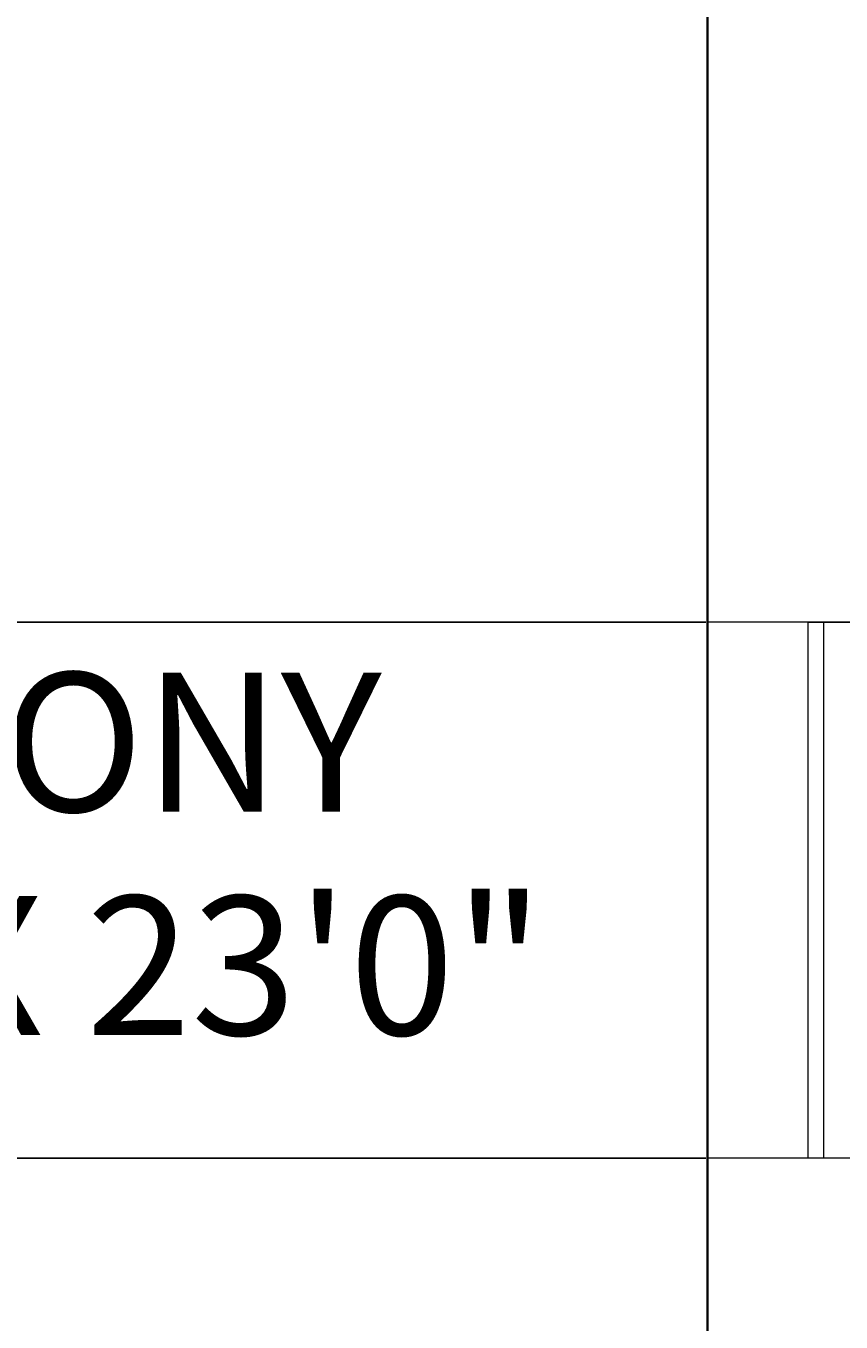
# Model space of a CAD drawing. Units: inches. Extents: x -61 to 1599, y -1316 to 257.
# Tile 58 of 204: x 48 to 85, y -282 to -224. Entities that reach past the tile are written whole.
import ezdxf

# ---------------------------------------------------------------- set-up
doc = ezdxf.new("R2010")
doc.units = ezdxf.units.IN
doc.header["$MEASUREMENT"] = 0
for name, color, linetype, lineweight in [('A-ANNO-DIMS', 2, 'Continuous', 18), ('A-AREA-IDEN', 1, 'Continuous', 18), ('WALLS', 4, 'Continuous', 35), ('WINDOWS', 220, 'Continuous', 18)]:
    doc.layers.add(name, color=color, linetype=linetype, lineweight=lineweight)
doc.styles.get("Standard").update_dxf_attribs({"font": 'arial.ttf'})
doc.dimstyles.get("Standard").update_dxf_attribs({"dimtxt": 0.18, "dimasz": 0.18, "dimexe": 0.18, "dimexo": 0.0625, "dimgap": 0.09, "dimtad": 0, "dimtih": 1, "dimtoh": 1, "dimdec": 0, "dimzin": 0, "dimdsep": 46, "dimlunit": 3, "dimtxsty": 'Standard', "dimcen": 0.09, "dimadec": 0, "dimazin": 0, "dimtfac": 1, "dimtdec": 0, "dimtofl": 0, "dimtmove": 0, "dimatfit": 3, "dimfxl": 1, "dimtolj": 1, "dimtzin": 0, "dimarcsym": 0})

# ---------------------------------------------------------------- blocks, each defined once
blk = doc.blocks.new('WIN-24IN')
for p, q in [((0, 4.5), (0, 9)), ((0, 9), (0, 0)), ((24, 9), (24, 0)), ((0, 5.192), (24, 5.192)), ((0, 4.5), (24, 4.5))]:
    blk.add_line(p, q)
blk = doc.blocks.new('*D687')
at = {"layer": 'A-ANNO-DIMS', "color": 0, "lineweight": -2, "transparency": 16777216}
for p, q in [((289.418, 181.677), (-61.077, 181.677)), ((-60.897, 181.497), (-60.897, -528.952)), ((-60.897, -1239.765), (-60.897, -529.316)), ((319.64, -1239.945), (-61.077, -1239.945))]:
    blk.add_line(p, q, dxfattribs=at)
at = {"layer": 'A-ANNO-DIMS', "color": 0, "transparency": 16777216}
for points in [[(-60.927, 181.497), (-60.867, 181.497), (-60.897, 181.677)], [(-60.927, -1239.765), (-60.867, -1239.765), (-60.897, -1239.945)]]:
    blk.add_solid(points, dxfattribs=at)
at = {"layer": 'DEFPOINTS', "color": 0, "transparency": 16777216}
for p in [(289.481, 181.677), (-60.897, -1239.945), (319.703, -1239.945)]:
    blk.add_point(p, dxfattribs=at)
at = {"layer": 'A-ANNO-DIMS', "color": 0, "transparency": 16777216, "insert": (-60.897, -529.134), "char_height": 0.18, "attachment_point": 5}
blk.add_mtext('\\A1;1421.6', dxfattribs=at)
blk = doc.blocks.new('*D699')
at = {"layer": 'A-ANNO-DIMS', "color": 0, "lineweight": -2, "transparency": 16777216}
for p, q in [((835.64, -167.169), (-61.077, -167.169)), ((-60.897, -167.349), (-60.897, -306.726)), ((-60.897, -446.466), (-60.897, -307.09)), ((841.64, -446.646), (-61.077, -446.646))]:
    blk.add_line(p, q, dxfattribs=at)
at = {"layer": 'A-ANNO-DIMS', "color": 0, "transparency": 16777216}
for points in [[(-60.927, -167.349), (-60.867, -167.349), (-60.897, -167.169)], [(-60.927, -446.466), (-60.867, -446.466), (-60.897, -446.646)]]:
    blk.add_solid(points, dxfattribs=at)
at = {"layer": 'DEFPOINTS', "color": 0, "transparency": 16777216}
for p in [(835.703, -167.169), (-60.897, -446.646), (841.703, -446.646)]:
    blk.add_point(p, dxfattribs=at)
at = {"layer": 'A-ANNO-DIMS', "color": 0, "transparency": 16777216, "insert": (-60.897, -306.908), "char_height": 0.18, "attachment_point": 5}
blk.add_mtext('\\A1;279.5', dxfattribs=at)
blk = doc.blocks.new('*D700')
at = {"layer": 'A-ANNO-DIMS', "color": 0, "lineweight": -2, "transparency": 16777216}
for p, q in [((14.703, -616.882), (14.703, 257.457)), ((14.883, 257.277), (96.772, 257.277)), ((179.572, 257.277), (97.683, 257.277)), ((179.752, -616.882), (179.752, 257.457))]:
    blk.add_line(p, q, dxfattribs=at)
at = {"layer": 'A-ANNO-DIMS', "color": 0, "transparency": 16777216}
for points in [[(14.883, 257.307), (14.883, 257.247), (14.703, 257.277)], [(179.572, 257.307), (179.572, 257.247), (179.752, 257.277)]]:
    blk.add_solid(points, dxfattribs=at)
at = {"layer": 'DEFPOINTS', "color": 0, "transparency": 16777216}
for p in [(179.752, 257.277), (14.703, -616.945), (179.752, -616.945)]:
    blk.add_point(p, dxfattribs=at)
at = {"layer": 'A-ANNO-DIMS', "color": 0, "transparency": 16777216, "insert": (97.227, 257.277), "char_height": 0.18, "attachment_point": 5}
blk.add_mtext('\\A1;165.05', dxfattribs=at)
blk = doc.blocks.new('*D706')
at = {"layer": 'A-ANNO-DIMS', "color": 0, "lineweight": -2, "transparency": 16777216}
for p, q in [((78.64, -175.323), (-61.077, -175.323)), ((-60.897, -175.503), (-60.897, -212.976)), ((-60.897, -250.814), (-60.897, -213.34)), ((78.64, -250.994), (-61.077, -250.994))]:
    blk.add_line(p, q, dxfattribs=at)
at = {"layer": 'A-ANNO-DIMS', "color": 0, "transparency": 16777216}
for points in [[(-60.927, -175.503), (-60.867, -175.503), (-60.897, -175.323)], [(-60.927, -250.814), (-60.867, -250.814), (-60.897, -250.994)]]:
    blk.add_solid(points, dxfattribs=at)
at = {"layer": 'DEFPOINTS', "color": 0, "transparency": 16777216}
for p in [(-60.897, -175.323), (78.703, -175.323), (78.703, -250.994)]:
    blk.add_point(p, dxfattribs=at)
at = {"layer": 'A-ANNO-DIMS', "color": 0, "transparency": 16777216, "insert": (-60.897, -213.158), "char_height": 0.18, "attachment_point": 5}
blk.add_mtext('\\A1;75.67', dxfattribs=at)
blk = doc.blocks.new('*D707')
at = {"layer": 'A-ANNO-DIMS', "color": 0, "lineweight": -2, "transparency": 16777216}
for p, q in [((78.64, -274.994), (-61.077, -274.994)), ((-60.897, -275.174), (-60.897, -308.474)), ((-60.897, -342.139), (-60.897, -308.838)), ((78.64, -342.319), (-61.077, -342.319))]:
    blk.add_line(p, q, dxfattribs=at)
at = {"layer": 'A-ANNO-DIMS', "color": 0, "transparency": 16777216}
for points in [[(-60.927, -275.174), (-60.867, -275.174), (-60.897, -274.994)], [(-60.927, -342.139), (-60.867, -342.139), (-60.897, -342.319)]]:
    blk.add_solid(points, dxfattribs=at)
at = {"layer": 'DEFPOINTS', "color": 0, "transparency": 16777216}
for p in [(78.703, -274.994), (-60.897, -342.319), (78.703, -342.319)]:
    blk.add_point(p, dxfattribs=at)
at = {"layer": 'A-ANNO-DIMS', "color": 0, "transparency": 16777216, "insert": (-60.897, -308.656), "char_height": 0.18, "attachment_point": 5}
blk.add_mtext('\\A1;67.33', dxfattribs=at)

msp = doc.modelspace()

# ---------------------------------------------------------------- linework, layer by layer
at = {"layer": 'WALLS'}
msp.add_line((78.7028, -175.3229), (78.7028, -432.3229), dxfattribs=at)

# ---------------------------------------------------------------- block references
at = {"layer": 'WINDOWS', "rotation": 270.0000000000001}
msp.add_blockref('WIN-24IN', (78.7027, -250.9933), dxfattribs=at)

# ---------------------------------------------------------------- texts
at = {"layer": 'A-AREA-IDEN'}
for s, height, p in [('BALCONY', 6.22364, (26.4051, -259.4795)), ('4\'7" X 23\'0"', 6.223643, (26.4051, -269.4772))]:
    msp.add_text(s, height=height, dxfattribs=at).set_placement(p)

# ---------------------------------------------------------------- dimensions: what is measured, and where the dimension line sits
at = {"layer": 'A-ANNO-DIMS'}
dim = msp.add_linear_dim(base=(179.7521, 257.2771), p1=(14.7028, -616.9446), p2=(179.7521, -616.9446), dimstyle='Standard', override={"dimdec": 2, "dimlfac": 1, "dimrnd": 0, "dimzin": 0, "dimdsep": 46, "dimlunit": 2}, dxfattribs=at)
dim.commit()
dim.dimension.update_dxf_attribs({"geometry": '*D700', "text_midpoint": (97.2274, 257.2771)})
for base, p1, p2, override, picture, middle in [((-60.8972, -1239.9446), (289.4807, 181.6771), (319.7028, -1239.9446), {"dimdec": 1, "dimlfac": 1, "dimrnd": 0, "dimzin": 0, "dimdsep": 46, "dimlunit": 2}, '*D687', (-60.8972, -529.1337)), ((-60.8972, -446.6462), (835.7028, -167.169), (841.7028, -446.6462), {"dimdec": 1, "dimlfac": 1, "dimrnd": 0, "dimzin": 0, "dimdsep": 46, "dimlunit": 2}, '*D699', (-60.8972, -306.9076)), ((-60.8972, -175.3229), (78.7028, -250.9938), (78.7028, -175.3229), {"dimdec": 2, "dimlfac": 1, "dimrnd": 0, "dimzin": 0, "dimdsep": 46, "dimlunit": 2}, '*D706', (-60.8972, -213.1583)), ((-60.8972, -342.3189), (78.7028, -274.9938), (78.7028, -342.3189), {"dimdec": 2, "dimlfac": 1, "dimrnd": 0, "dimzin": 0, "dimdsep": 46, "dimlunit": 2}, '*D707', (-60.8972, -308.6563))]:
    dim = msp.add_linear_dim(base=base, p1=p1, p2=p2, angle=90, dimstyle='Standard', override=override, dxfattribs=at)
    dim.commit()
    dim.dimension.update_dxf_attribs({"geometry": picture, "text_midpoint": middle})

doc.saveas('drawing.dxf')
